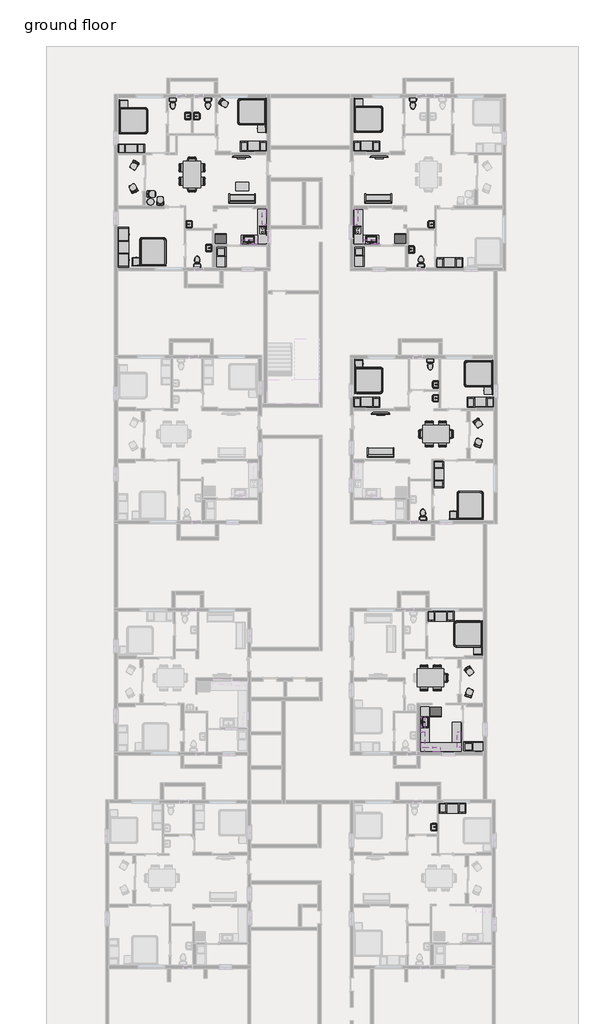
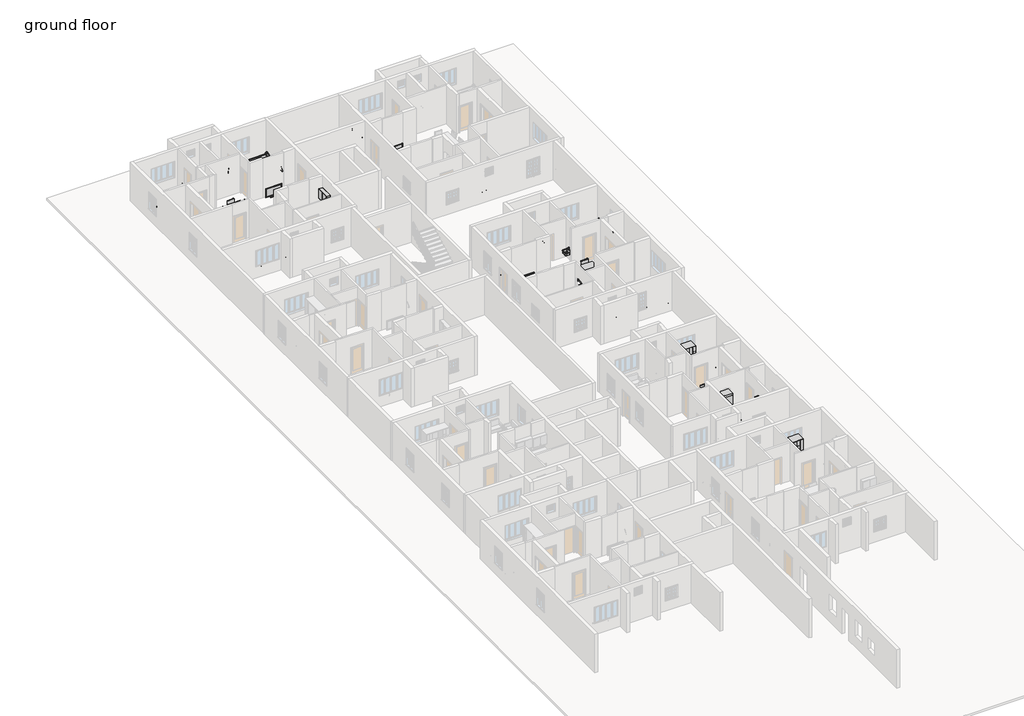
# One storey, part 13 of 16: 81 furniture elements, 19 flow terminals, 11 proxies.
# Revit data of these elements (continued)
# Elements 50, 51, 52, 53, 54, 55, 56, 57, 58, 59, 60, 61 (IfcFurniture, "Chair-Task : Chair-Task")
#   Phase Created = New Construction
#   Materials on its faces: "Plastic - Black", "Textile - Slate Blue"
# Elements 62, 63, 64, 65, 66 (IfcFurniture, "Chair-Task Arms : Chair-Task Arms")
#   Phase Created = New Construction
#   Materials on its faces: "Plastic - Black", "Textile - Slate Blue"
# Elements 67, 68 (IfcFurniture, "Counter Top : 24\" Depth")
#   Length = 8' - 0"
#   Phase Created = New Construction
#   Materials on its faces: "Counter Top"
# Element 69 (IfcFurniture, "Counter Top : 24\" Depth")
#   Length = 9' - 4 1/2"
#   Phase Created = New Construction
#   Materials on its faces: "Counter Top"
# Element 70 (IfcFurniture, "Counter Top : 24\" Depth")
#   Length = 4' - 8.10552"
#   Phase Created = New Construction
#   Materials on its faces: "Counter Top"
# Elements 71, 72 (IfcFurniture, "Counter Top w Sink Hole : 24\" Depth")
#   Sink Opening Width = 2' - 3"
#   Sink Opening Depth = 1' - 3"
#   Sink Location To Wall = 0' - 6"
#   Sink Location = 2' - 0"
#   Length = 3' - 8.18593"
#   Phase Created = New Construction
#   Materials on its faces: "Counter Top"
# Element 73 (IfcFurniture, "Counter Top w Sink Hole : 24\" Depth")
#   Sink Opening Width = 2' - 3"
#   Sink Opening Depth = 1' - 3"
#   Sink Location To Wall = 0' - 6"
#   Sink Location = 4' - 8 1/8"
#   Length = 8' - 2"
#   Phase Created = New Construction
#   Materials on its faces: "Counter Top"
# Elements 74, 75, 76, 77, 78, 79, 80, 81, 82 (IfcFurniture, "Entertainment Center : 72\" x 72\" x 24\"")
#   Phase Created = New Construction
#   Materials on its faces: "Steel, Chrome Plated", "Glass - Clear, Grey"
# Element 83 (IfcFurniture, "Entertainment Center : 96\" x 84\" x 30\"")
#   Phase Created = New Construction
#   Materials on its faces: "Laminate, Ivory, Matte", "Steel, Chrome Plated", "Glass - Clear, Grey"
# Elements 84, 85, 86, 87, 88, 89, 90, 91, 92 (IfcFurniture, "Seating-Auditorium : 18\" x 24\" x 30\"")
#   Phase Created = New Construction
#   Materials on its faces: "Steel, Paint Finish, Dark Gray, Matte", "Linen, Beige"
# Elements 93, 94, 95 (IfcFurniture, "Sofa : 72\"")
#   Phase Created = New Construction
#   Materials on its faces: "Cherry", "Linen, Beige"
# Elements 96, 97, 98 (IfcFurniture, "TV - Flat Screen : 50\"")
#   Stand = yes
#   Phase Created = New Construction
#   Materials on its faces: "TV - Black", "TV - Glass", "TV - Screen"
# Element 99 (IfcFurniture, "Table-Coffee Rectangular : 48\" x 24\"")
#   Phase Created = New Construction
#   Materials on its faces: "Metal - Chrome", "Laminate - Ivory,Matte"
# Elements 100, 101 (IfcFurniture, "Table-Conference2 w Chairs : 48\" x 144\"")
#   Phase Created = New Construction
#   Materials on its faces: "Wood - Cherry"
# Element 102 (IfcFurniture, "Table-Conference2 w Chairs : dining table")
#   Phase Created = New Construction
#   Materials on its faces: "Wood - Cherry"
# Element 103 (IfcFurniture, "Table-Trio End : 20\" Diameter")
#   Phase Created = New Construction
#   Materials on its faces: "Wood - Birch", "Laminate - Ivory,Matte"
# Elements 104, 105, 106, 107, 108, 109, 110, 111 (IfcFurniture, "Upper Cabinet-Double Door-Wall : 42\"")
#   Phase Created = New Construction
#   Materials on its faces: "Cabinets - Handles", "Cabinet"
# Materials
#   "Metal - Chrome": colour RGB 57 57 57, transparency 0
#   "Metal - Steel, Polished": colour RGB 57 57 57, transparency 0
#   "Metal - Paint Finish - Ivory,Glossy": colour RGB 247 247 239, transparency 0
#   "Metal - Paint Finish - Ivory,Matte": colour RGB 247 247 239, transparency 0
#   "Steel, Polished": class "Metal", colour RGB 192 192 192, transparency 0, Description = "Polished steel", Cost = 0
#   "Porcelain, Linen": class "Ceramic", colour RGB 249 239 230, transparency 0, Description = "Porcelain, linen", Cost = 0
#   "Laminate, Linen, Matte": class "Plastic", colour RGB 249 239 230, transparency 0, Description = "Plastic Laminate - Linen, Matte", Cost = 0
#   "Cabinets": colour RGB 249 249 249, transparency 0
#   "Cabinets - Handles": colour RGB 57 57 57, transparency 0
#   "Plastic - Black": colour RGB 0 0 0, transparency 0.7
#   "Textile - Slate Blue": colour RGB 98 102 118, transparency 0
#   "Laminate, Ivory, Matte": class "Plastic", colour RGB 247 247 239, transparency 0, Description = "Plastic Laminate - Ivory, Matte", Cost = 0
#   "Linen, Beige": class "Textile", colour RGB 249 239 230, transparency 0, Description = "Linen, beige", Cost = 0
#   "Steel, Paint Finish, Dark Gray, Matte": class "Metal", colour RGB 0 0 0, transparency 0, Description = "Steel, paint finish, dark gray, matte", Cost = 0
#   "Cherry": class "Wood", colour RGB 226 177 128, transparency 0, Description = "Prunus Serotina", Cost = 0
#   "Laminate - Ivory,Matte": colour RGB 127 127 127, transparency 0
#   "Wood - Cherry": colour RGB 151 75 0, transparency 0
#   "Wood - Birch": colour RGB 230 196 162, transparency 0
#   "wood 2": class "Wood", colour RGB 196 146 67, transparency 0
#   "ss": class "Metal", colour RGB 189 187 185, transparency 0
#   "new wood": class "Wood", colour RGB 133 62 31, transparency 0
#   "fabric 2": class "Fabric", colour RGB 198 193 133, transparency 0
#   "wood light": class "Wood", colour RGB 198 165 122, transparency 0
#   "fabric": class "Fabric", colour RGB 198 193 133, transparency 0
#   "Cabinet": colour RGB 204 122 2, transparency 0
#   "Counter Top": class "Wood", colour RGB 226 177 128, transparency 0
#   "Steel, Chrome Plated": class "Metal", colour RGB 17 17 17, transparency 0, Description = "Chromiuim plated steel", Cost = 0
#   "Glass - Clear, Grey": class "Glass", colour RGB 252 255 255, transparency 0.64
#   "TV - Black": colour RGB 49 49 49, transparency 0
#   "TV - Glass": colour RGB 157 157 157, transparency 0.9
#   "TV - Screen": colour RGB 0 0 0, transparency 0
